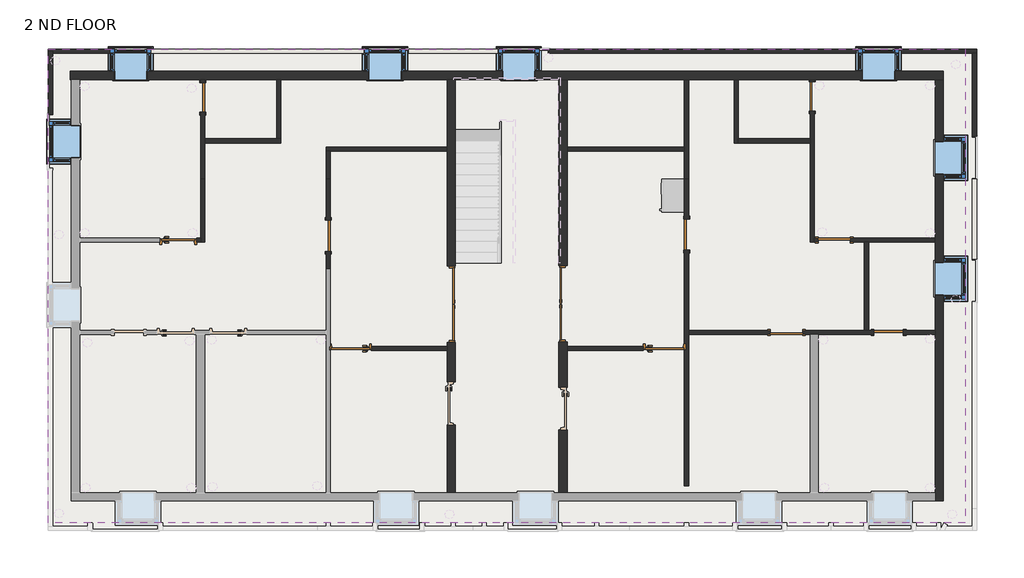
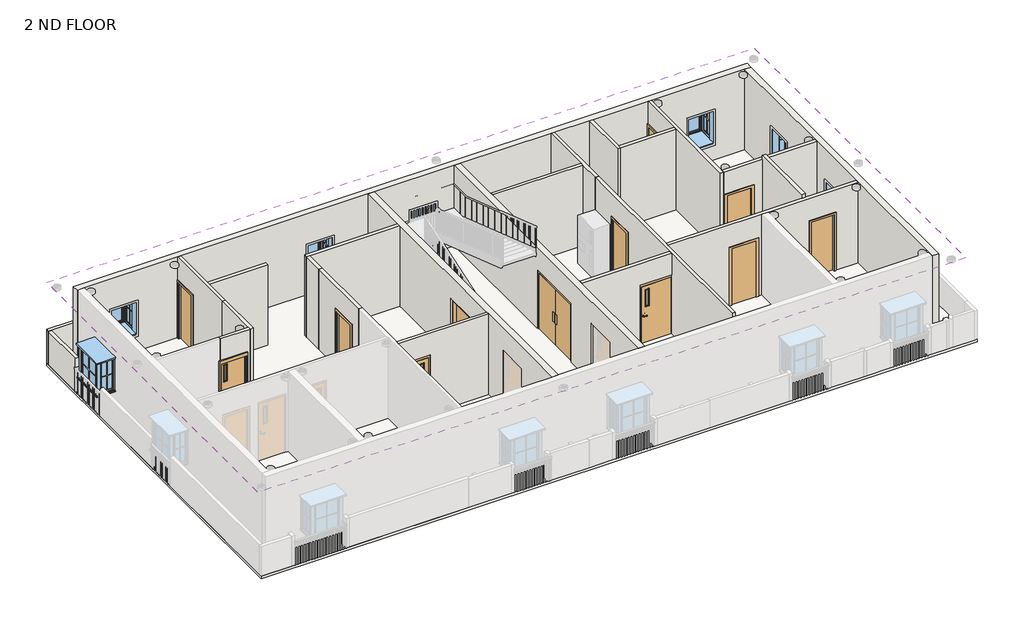
# One storey, part 2 of 7: 32 walls, 12 doors, 7 windows, 1 covering, 1 slab.
"""IFC4 building model written with IfcOpenShell, lengths in millimetres."""

from ifc_helpers import new_model, si_unit, frame, origin, place, context, project, spatial, polyline, outline, extrude, faceted_brep, transform, mapped, element, save
from components import door_2c854dd0, door_cf1f2706, door_4f5842df, door_passage_single_vision_lite_3_x7_440dd290, door_70e57c00, door_700d3439, door_8cb1b8a7, door_38851409, door_d141acb4, window_bay_casement_box_90_degree_angle_center_fixed_4_x3_2dea7aab

model = new_model("IFC4")

# Units and contexts
model_context = context("Model", 3, world=origin())
ifc_project = project(units=[si_unit("LENGTHUNIT", "METRE", prefix="MILLI")], contexts=[model_context])

# Site, building, storey
site = spatial("IfcSite", under=ifc_project)
building = spatial("IfcBuilding", under=site)
storey = spatial("IfcBuildingStorey", under=building, Name="2 ND FLOOR", Elevation=6400.8)

# Covering
placement = place(None, origin())
element("IfcCovering", 1, ObjectType="2' x 4' ACT System", at=placement, inside=storey, context=model_context, shape_type="SweptSolid", body=[
    extrude(outline(polyline([(12235.5012075, 8470.0067329), (12235.5012075, -4623.6932193), (-13088.8067989, -4623.6932193), (-13088.8067989, 8470.0067329), (12235.5012075, 8470.0067329)])), frame((0.0, 0.0, 9448.8), z_axis=(0.0, 0.0, 1.0), x_axis=(1.0, 0.0, 0.0)), (0.0, 0.0, 1.0), 57.15),
])

# Doors
door_shape = door_2c854dd0(model_context)
element("IfcDoor", 2, ObjectType="Door-Passage-Double-Flush-Dbl_Acting : 6'79\" X 84\"", at=placement, inside=storey, context=model_context, shape_type="MappedRepresentation", body=[
    mapped(door_shape, transform((-1969.4487998, 1424.4578621, 6400.8), x_axis=(0.0, -1.0, 0.0), y_axis=(1.0, 0.0, 0.0), z_axis=(0.0, 0.0, 1.0))),
])
element("IfcDoor", 3, ObjectType="Door-Passage-Double-Flush-Dbl_Acting : 6'79\" X 84\"", at=placement, inside=storey, context=model_context, shape_type="MappedRepresentation", body=[
    mapped(door_shape, transform((1128.8432011, 1434.2067807, 6400.8), x_axis=(0.0, 1.0, 0.0), y_axis=(-1.0, 0.0, 0.0), z_axis=(0.0, 0.0, 1.0))),
])
door_2_shape = door_cf1f2706(model_context)
element("IfcDoor", 4, ObjectType="Door-Passage-Single-Vision_Lite : 3'6\"X7' 2", at=placement, inside=storey, context=model_context, shape_type="MappedRepresentation", body=[
    mapped(door_2_shape, transform((-4750.7487995, 211.6078621, 6400.8), x_axis=(-1.0, 0.0, 0.0), y_axis=(0.0, -1.0, 0.0), z_axis=(0.0, 0.0, 1.0))),
])
door_3_shape = door_4f5842df(model_context)
element("IfcDoor", 5, ObjectType="Door-Passage-Single-Vision_Lite : 3'6\"X7' 2", at=placement, inside=storey, context=model_context, shape_type="MappedRepresentation", body=[
    mapped(door_3_shape, transform((3923.3512082, 211.6078621, 6400.8), x_axis=(1.0, 0.0, 0.0), y_axis=(0.0, 1.0, 0.0), z_axis=(0.0, 0.0, 1.0))),
])
door_passage_single_vision_lite_3_x7_shape = door_passage_single_vision_lite_3_x7_440dd290(model_context)
element("IfcDoor", 6, ObjectType="Door-Passage-Single-Vision_Lite : 3'X7'", at=placement, inside=storey, context=model_context, shape_type="MappedRepresentation", body=[
    mapped(door_passage_single_vision_lite_3_x7_shape, transform((-9501.8462614, 3186.8067332, 6400.8), x_axis=(1.0, 0.0, 0.0), y_axis=(0.0, 1.0, 0.0), z_axis=(0.0, 0.0, 1.0))),
])
door_4_shape = door_70e57c00(model_context)
element("IfcDoor", 7, ObjectType="Single-Flush : 2'10\" x 7'", at=placement, inside=storey, context=model_context, shape_type="MappedRepresentation", body=[
    mapped(door_4_shape, transform((-5360.3487995, 3313.8067802, 6400.8), x_axis=(0.0, -1.0, 0.0), y_axis=(1.0, 0.0, 0.0), z_axis=(0.0, 0.0, 1.0))),
])
door_5_shape = door_700d3439(model_context)
element("IfcDoor", 8, ObjectType="Single-Flush : 2'10\" x 7'", at=placement, inside=storey, context=model_context, shape_type="MappedRepresentation", body=[
    mapped(door_5_shape, transform((4532.9512082, 3351.906733, 6400.8), x_axis=(0.0, -1.0, 0.0), y_axis=(1.0, 0.0, 0.0), z_axis=(0.0, 0.0, 1.0))),
])
door_6_shape = door_8cb1b8a7(model_context)
element("IfcDoor", 9, ObjectType="Single-Flush : 2'11\"x 7'", at=placement, inside=storey, context=model_context, shape_type="MappedRepresentation", body=[
    mapped(door_6_shape, transform((8609.6512079, 3193.1567332, 6400.8), x_axis=(-1.0, 0.0, 0.0), y_axis=(0.0, -1.0, 0.0), z_axis=(0.0, 0.0, 1.0))),
])
element("IfcDoor", 10, ObjectType="Single-Flush : 2'11\"x 7'", at=placement, inside=storey, context=model_context, shape_type="MappedRepresentation", body=[
    mapped(door_6_shape, transform((7295.2012079, 640.4567334, 6400.8), x_axis=(1.0, 0.0, 0.0), y_axis=(0.0, 1.0, 0.0), z_axis=(0.0, 0.0, 1.0))),
])
door_7_shape = door_38851409(model_context)
element("IfcDoor", 11, ObjectType="Single-Flush : 2'8\"x 7'", at=placement, inside=storey, context=model_context, shape_type="MappedRepresentation", body=[
    mapped(door_7_shape, transform((-8827.4487992, 7136.5067329, 6400.8), x_axis=(0.0, 1.0, 0.0), y_axis=(-1.0, 0.0, 0.0), z_axis=(0.0, 0.0, 1.0))),
])
element("IfcDoor", 12, ObjectType="Single-Flush : 2'8\"x 7'", at=placement, inside=storey, context=model_context, shape_type="MappedRepresentation", body=[
    mapped(door_7_shape, transform((10111.5098918, 640.4567334, 6400.8), x_axis=(-1.0, 0.0, 0.0), y_axis=(0.0, -1.0, 0.0), z_axis=(0.0, 0.0, 1.0))),
])
door_8_shape = door_d141acb4(model_context)
element("IfcDoor", 13, ObjectType="Single-Flush : 2'8\"x 7'", at=placement, inside=storey, context=model_context, shape_type="MappedRepresentation", body=[
    mapped(door_8_shape, transform((8000.0512079, 7167.840939, 6400.8), x_axis=(0.0, 1.0, 0.0), y_axis=(-1.0, 0.0, 0.0), z_axis=(0.0, 0.0, 1.0))),
])

# Slab
element("IfcSlab", 14, ObjectType="LW Concrete on Metal Deck", at=placement, inside=storey, context=model_context, shape_type="SweptSolid", body=[
    extrude(outline(polyline([(12540.3012043, 8470.0067329), (12540.3012043, -4826.8932661), (-13088.8067989, -4826.8932661), (-13088.8067989, 8470.0067329), (12540.3012043, 8470.0067329)])), frame((0.0, 0.0, 6296.025), z_axis=(0.0, 0.0, 1.0), x_axis=(1.0, 0.0, 0.0)), (0.0, 0.0, 1.0), 104.775),
])

# Walls
element("IfcWall", 15, ObjectType="Generic - 4.5\"", at=placement, inside=storey, context=model_context, shape_type="Brep", body=[
    faceted_brep([(-8884.5987992, 4875.906733, 6400.8), (-8884.5987992, 3250.3067332, 6400.8), (-8884.5987992, 3136.0067332, 6400.8), (-8884.5987992, 3136.0067332, 9448.8), (-8884.5987992, 3250.3067332, 9448.8), (-8884.5987992, 4875.906733, 9448.8), (-8770.2987992, 4875.906733, 6400.8), (-8770.2987992, 4875.906733, 9448.8), (-8770.2987992, 3136.0067332, 9448.8), (-8770.2987992, 3136.0067332, 6400.8)], [[[0, 1, 2, 3, 4, 5]], [[6, 7, 8, 9]], [[2, 1, 0, 6, 9]], [[5, 4, 3, 8, 7]], [[0, 5, 7, 6]], [[3, 2, 9, 8]]]),
])
element("IfcWall", 16, ObjectType="Generic - 4.5\"", at=placement, inside=storey, context=model_context, shape_type="SweptSolid", body=[
    extrude(outline(polyline([(9448.8, -2077.3987998), (9448.8, -5303.1987995), (8636.0, -5303.1987995), (8636.0, -4166.5487995), (6400.8, -4166.5487995), (6400.8, -2077.3987998), (9448.8, -2077.3987998)])), frame((0.0, 148.1078621, 0.0), z_axis=(0.0, 1.0, 0.0), x_axis=(0.0, 0.0, 1.0)), (0.0, 0.0, 1.0), 114.3),
])
element("IfcWall", 17, ObjectType="Generic - 4.5\"", at=placement, inside=storey, context=model_context, shape_type="Brep", body=[
    faceted_brep([(-2077.3987998, 5764.9067329, 6400.8), (-5417.4987995, 5764.9067329, 6400.8), (-5417.4987995, 5764.9067329, 9448.8), (-2077.3987998, 5764.9067329, 9448.8), (-2077.3987998, 5650.6067329, 6400.8), (-2077.3987998, 5650.6067329, 9448.8), (-5303.1987995, 5650.6067329, 9448.8), (-5417.4987995, 5650.6067329, 9448.8), (-5417.4987995, 5650.6067329, 6400.8), (-5303.1987995, 5650.6067329, 6400.8)], [[[0, 1, 2, 3]], [[4, 5, 6, 7, 8, 9]], [[1, 0, 4, 9, 8]], [[3, 2, 7, 6, 5]], [[2, 1, 8, 7]], [[0, 3, 5, 4]]]),
])
element("IfcWall", 18, ObjectType="Generic - 4.5\"", at=placement, inside=storey, context=model_context, shape_type="SweptSolid", body=[
    extrude(outline(polyline([(-5417.4987995, 4875.90678), (-5417.4987995, 5650.6067329), (-5303.1987995, 5650.6067329), (-5303.1987995, 4875.90678), (-5417.4987995, 4875.90678)])), frame((0.0, 0.0, 6400.8), z_axis=(0.0, 0.0, 1.0), x_axis=(1.0, 0.0, 0.0)), (0.0, 0.0, 1.0), 3048.0),
])
element("IfcWall", 19, ObjectType="Generic - 4.5\"", at=placement, inside=storey, context=model_context, shape_type="SweptSolid", body=[
    extrude(outline(polyline([(4475.8012082, 5650.6067329), (1250.0012085, 5650.6067329), (1250.0012085, 5764.9067329), (4475.8012082, 5764.9067329), (4475.8012082, 5650.6067329)])), frame((0.0, 0.0, 6400.8), z_axis=(0.0, 0.0, 1.0), x_axis=(1.0, 0.0, 0.0)), (0.0, 0.0, 1.0), 3048.0),
])
element("IfcWall", 20, ObjectType="Generic - 4.5\"", at=placement, inside=storey, context=model_context, shape_type="Brep", body=[
    faceted_brep([(4475.8012082, 7631.8067329, 6400.8), (4475.8012082, 5764.9067329, 6400.8), (4475.8012082, 5650.6067329, 6400.8), (4475.8012082, 4875.906733, 6400.8), (4475.8012082, 4875.906733, 9448.8), (4475.8012082, 5650.6067329, 9448.8), (4475.8012082, 5764.9067329, 9448.8), (4475.8012082, 7631.8067329, 9448.8), (4590.1012082, 7631.8067329, 6400.8), (4590.1012082, 7631.8067329, 9448.8), (4590.1012082, 4875.906733, 9448.8), (4590.1012082, 4875.906733, 6400.8)], [[[0, 1, 2, 3, 4, 5, 6, 7]], [[8, 9, 10, 11]], [[3, 2, 1, 0, 8, 11]], [[4, 3, 11, 10]], [[7, 6, 5, 4, 10, 9]], [[0, 7, 9, 8]]]),
])
element("IfcWall", 21, ObjectType="Generic - 4.5\"", at=placement, inside=storey, context=model_context, shape_type="Brep", body=[
    faceted_brep([(4475.8012082, -3594.9932193, 6400.8), (4475.8012082, -3594.9932193, 9448.8), (4475.8012082, 148.1078621, 9448.8), (4475.8012082, 262.4078621, 9448.8), (4475.8012082, 4875.906733, 9448.8), (4475.8012082, 4875.906733, 6400.8), (4475.8012082, 3783.706733, 6400.8), (4475.8012082, 3783.706733, 8534.4), (4475.8012082, 2920.106733, 8534.4), (4475.8012082, 2920.106733, 6400.8), (4475.8012082, 262.4078621, 6400.8), (4475.8012082, 262.4078621, 8636.0), (4475.8012082, 148.1078621, 8636.0), (4475.8012082, 148.1078621, 6400.8), (4590.1012082, -3594.9932193, 9448.8), (4590.1012082, -3594.9932193, 6400.8), (4590.1012082, 583.3067334, 6400.8), (4590.1012082, 697.6067334, 6400.8), (4590.1012082, 2920.106733, 6400.8), (4590.1012082, 2920.106733, 8534.4), (4590.1012082, 3783.706733, 8534.4), (4590.1012082, 3783.706733, 6400.8), (4590.1012082, 4875.906733, 6400.8), (4590.1012082, 4875.906733, 9448.8), (4590.1012082, 697.6067334, 9448.8), (4590.1012082, 583.3067334, 9448.8), (4507.5512082, 148.1078621, 6400.8), (4507.5512082, 262.4078621, 6400.8), (4507.5512082, 148.1078621, 8636.0), (4507.5512082, 262.4078621, 8636.0)], [[[0, 1, 2, 3, 4, 5, 6, 7, 8, 9, 10, 11, 12, 13]], [[14, 15, 16, 17, 18, 19, 20, 21, 22, 23, 24, 25]], [[15, 0, 13, 26, 27, 10, 9, 18, 17, 16]], [[5, 22, 21, 6]], [[1, 0, 15, 14]], [[4, 3, 2, 1, 14, 25, 24, 23]], [[5, 4, 23, 22]], [[19, 18, 9, 8]], [[20, 19, 8, 7]], [[21, 20, 7, 6]], [[28, 26, 13, 12]], [[27, 29, 11, 10]], [[26, 28, 29, 27]], [[29, 28, 12, 11]]]),
])
element("IfcWall", 22, ObjectType="Generic - 4.5\"", at=placement, inside=storey, context=model_context, shape_type="Brep", body=[
    faceted_brep([(5847.401208, 7631.8067329, 6400.8), (5847.401208, 5879.2067329, 6400.8), (5847.401208, 5879.2067329, 9448.8), (5847.401208, 7631.8067329, 9448.8), (5961.701208, 7631.8067329, 6400.8), (5961.701208, 7631.8067329, 9448.8), (5961.701208, 5993.5067329, 9448.8), (5961.701208, 5879.2067329, 9448.8), (5961.701208, 5879.2067329, 6400.8), (5961.701208, 5993.5067329, 6400.8)], [[[0, 1, 2, 3]], [[4, 5, 6, 7, 8, 9]], [[1, 0, 4, 9, 8]], [[3, 2, 7, 6, 5]], [[0, 3, 5, 4]], [[2, 1, 8, 7]]]),
])
element("IfcWall", 23, ObjectType="Generic - 4.5\"", at=placement, inside=storey, context=model_context, shape_type="SweptSolid", body=[
    extrude(outline(polyline([(7942.9012079, 5879.2067329), (5961.701208, 5879.2067329), (5961.701208, 5993.5067329), (7942.9012079, 5993.5067329), (7942.9012079, 5879.2067329)])), frame((0.0, 0.0, 6400.8), z_axis=(0.0, 0.0, 1.0), x_axis=(1.0, 0.0, 0.0)), (0.0, 0.0, 1.0), 3048.0),
])
element("IfcWall", 24, ObjectType="Generic - 4.5\"", at=placement, inside=storey, context=model_context, shape_type="Brep", body=[
    faceted_brep([(7942.9012079, 7625.040939, 6400.8), (7942.9012079, 7574.240939, 6400.8), (7942.9012079, 7574.240939, 8534.4), (7942.9012079, 6761.440939, 8534.4), (7942.9012079, 6761.440939, 6400.8), (7942.9012079, 5993.5067329, 6400.8), (7942.9012079, 5879.2067329, 6400.8), (7942.9012079, 3136.0067332, 6400.8), (7942.9012079, 3136.0067332, 9448.8), (7942.9012079, 5879.2067329, 9448.8), (7942.9012079, 5993.5067329, 9448.8), (7942.9012079, 7625.040939, 9448.8), (8057.2012079, 7574.240939, 8534.4), (8057.2012079, 7574.240939, 6400.8), (8057.2012079, 7625.040939, 6400.8), (8057.2012079, 7625.040939, 9448.8), (8057.2012079, 3250.3067332, 9448.8), (8057.2012079, 3136.0067332, 9448.8), (8057.2012079, 3136.0067332, 6400.8), (8057.2012079, 3250.3067332, 6400.8), (8057.2012079, 6761.440939, 6400.8), (8057.2012079, 6761.440939, 8534.4)], [[[0, 1, 2, 3, 4, 5, 6, 7, 8, 9, 10, 11]], [[12, 13, 14, 15, 16, 17, 18, 19, 20, 21]], [[14, 13, 1, 0]], [[20, 19, 18, 7, 6, 5, 4]], [[11, 10, 9, 8, 17, 16, 15]], [[0, 11, 15, 14]], [[8, 7, 18, 17]], [[2, 1, 13, 12]], [[3, 2, 12, 21]], [[4, 3, 21, 20]]]),
])
element("IfcWall", 25, ObjectType="Generic - 4.5\"", at=placement, inside=storey, context=model_context, shape_type="Brep", body=[
    faceted_brep([(8165.1512079, 3250.3067332, 8534.4), (8165.1512079, 3250.3067332, 6400.8), (8057.2012079, 3250.3067332, 6400.8), (8057.2012079, 3250.3067332, 9448.8), (11397.3012075, 3250.3067332, 9448.8), (11397.3012075, 3250.3067332, 6400.8), (9054.1512079, 3250.3067332, 6400.8), (9054.1512079, 3250.3067332, 8534.4), (8057.2012079, 3136.0067332, 6400.8), (8165.1512079, 3136.0067332, 6400.8), (8165.1512079, 3136.0067332, 8534.4), (9054.1512079, 3136.0067332, 8534.4), (9054.1512079, 3136.0067332, 6400.8), (9438.4098918, 3136.0067332, 6400.8), (9565.4098918, 3136.0067332, 6400.8), (11397.3012075, 3136.0067332, 6400.8), (11397.3012075, 3136.0067332, 9448.8), (8057.2012079, 3136.0067332, 9448.8)], [[[0, 1, 2, 3, 4, 5, 6, 7]], [[8, 9, 10, 11, 12, 13, 14, 15, 16, 17]], [[6, 5, 15, 14, 13, 12]], [[2, 1, 9, 8]], [[4, 3, 17, 16]], [[3, 2, 8, 17]], [[5, 4, 16, 15]], [[10, 9, 1, 0]], [[11, 10, 0, 7]], [[12, 11, 7, 6]]]),
])
element("IfcWall", 26, ObjectType="Generic - 4.5\"", at=placement, inside=storey, context=model_context, shape_type="Brep", body=[
    faceted_brep([(7739.7012079, 583.3067334, 8534.4), (7739.7012079, 583.3067334, 6400.8), (7942.9012079, 583.3067334, 6400.8), (8171.5012079, 583.3067334, 6400.8), (9705.1098918, 583.3067334, 6400.8), (9705.1098918, 583.3067334, 8534.4), (10517.9098918, 583.3067334, 8534.4), (10517.9098918, 583.3067334, 6400.8), (11397.3012075, 583.3067334, 6400.8), (11397.3012075, 583.3067334, 9448.8), (8171.5012079, 583.3067334, 9448.8), (7942.9012079, 583.3067334, 9448.8), (4590.1012082, 583.3067334, 9448.8), (4590.1012082, 583.3067334, 6400.8), (6850.7012079, 583.3067334, 6400.8), (6850.7012079, 583.3067334, 8534.4), (9705.1098918, 697.6067334, 6400.8), (9565.4098918, 697.6067334, 6400.8), (9438.4098918, 697.6067334, 6400.8), (7739.7012079, 697.6067334, 6400.8), (7739.7012079, 697.6067334, 8534.4), (6850.7012079, 697.6067334, 8534.4), (6850.7012079, 697.6067334, 6400.8), (4590.1012082, 697.6067334, 6400.8), (4590.1012082, 697.6067334, 9448.8), (11397.3012075, 697.6067334, 9448.8), (11397.3012075, 697.6067334, 6400.8), (10517.9098918, 697.6067334, 6400.8), (10517.9098918, 697.6067334, 8534.4), (9705.1098918, 697.6067334, 8534.4)], [[[0, 1, 2, 3, 4, 5, 6, 7, 8, 9, 10, 11, 12, 13, 14, 15]], [[16, 17, 18, 19, 20, 21, 22, 23, 24, 25, 26, 27, 28, 29]], [[27, 26, 8, 7]], [[14, 13, 23, 22]], [[4, 3, 2, 1, 19, 18, 17, 16]], [[12, 11, 10, 9, 25, 24]], [[9, 8, 26, 25]], [[13, 12, 24, 23]], [[5, 4, 16, 29]], [[6, 5, 29, 28]], [[7, 6, 28, 27]], [[20, 19, 1, 0]], [[21, 20, 0, 15]], [[22, 21, 15, 14]]]),
])
element("IfcWall", 27, ObjectType="Generic - 4.5\"", at=placement, inside=storey, context=model_context, shape_type="Brep", body=[
    faceted_brep([(-8770.2987992, 7542.9067329, 8534.4), (-8770.2987992, 7542.9067329, 6400.8), (-8770.2987992, 7631.8067329, 6400.8), (-8770.2987992, 7631.8067329, 9448.8), (-8770.2987992, 5993.5067329, 9448.8), (-8770.2987992, 5879.2067329, 9448.8), (-8770.2987992, 4875.906733, 9448.8), (-8770.2987992, 4875.906733, 6400.8), (-8770.2987992, 5879.2067329, 6400.8), (-8770.2987992, 5993.5067329, 6400.8), (-8770.2987992, 6730.1067329, 6400.8), (-8770.2987992, 6730.1067329, 8534.4), (-8884.5987992, 7631.8067329, 6400.8), (-8884.5987992, 7542.9067329, 6400.8), (-8884.5987992, 7542.9067329, 8534.4), (-8884.5987992, 6730.1067329, 8534.4), (-8884.5987992, 6730.1067329, 6400.8), (-8884.5987992, 4875.906733, 6400.8), (-8884.5987992, 4875.906733, 9448.8), (-8884.5987992, 7631.8067329, 9448.8)], [[[0, 1, 2, 3, 4, 5, 6, 7, 8, 9, 10, 11]], [[12, 13, 14, 15, 16, 17, 18, 19]], [[2, 1, 13, 12]], [[10, 9, 8, 7, 17, 16]], [[6, 5, 4, 3, 19, 18]], [[7, 6, 18, 17]], [[3, 2, 12, 19]], [[14, 13, 1, 0]], [[15, 14, 0, 11]], [[16, 15, 11, 10]]]),
])
element("IfcWall", 28, ObjectType="Generic - 4.5\"", at=placement, inside=storey, context=model_context, shape_type="Brep", body=[
    faceted_brep([(-8770.2987992, 5879.2067329, 6400.8), (-6674.7987994, 5879.2067329, 6400.8), (-6674.7987994, 5879.2067329, 9448.8), (-8770.2987992, 5879.2067329, 9448.8), (-8770.2987992, 5993.5067329, 6400.8), (-8770.2987992, 5993.5067329, 9448.8), (-6674.7987994, 5993.5067329, 9448.8), (-6674.7987994, 5993.5067329, 7772.4), (-6674.7987994, 5993.5067329, 6400.8), (-6789.0987994, 5993.5067329, 6400.8)], [[[0, 1, 2, 3]], [[4, 5, 6, 7, 8, 9]], [[1, 0, 4, 9, 8]], [[3, 2, 6, 5]], [[0, 3, 5, 4]], [[2, 1, 8, 7, 6]]]),
])
element("IfcWall", 29, ObjectType="Generic - 4.5\"", at=placement, inside=storey, context=model_context, shape_type="SweptSolid", body=[
    extrude(outline(polyline([(-6674.7987994, 7631.8067329), (-6674.7987994, 5993.5067329), (-6789.0987994, 5993.5067329), (-6789.0987994, 7631.8067329), (-6674.7987994, 7631.8067329)])), frame((0.0, 0.0, 6400.8), z_axis=(0.0, 0.0, 1.0), x_axis=(1.0, 0.0, 0.0)), (0.0, 0.0, 1.0), 1371.6),
])
element("IfcWall", 30, ObjectType="Generic - 4.5\"", at=placement, inside=storey, context=model_context, shape_type="SweptSolid", body=[
    extrude(outline(polyline([(9448.8, -8884.5987992), (9448.8, -9959.0462614), (8636.0, -9959.0462614), (8636.0, -8993.8462614), (6400.8, -8993.8462614), (6400.8, -8884.5987992), (9448.8, -8884.5987992)])), frame((0.0, 3136.0067332, 0.0), z_axis=(0.0, 1.0, 0.0), x_axis=(0.0, 0.0, 1.0)), (0.0, 0.0, 1.0), 114.3),
])
element("IfcWall", 31, ObjectType="Generic - 4.5\"", at=placement, inside=storey, context=model_context, shape_type="SweptSolid", body=[
    extrude(outline(polyline([(2882.0067802, 8534.4), (2882.0067802, 6400.8), (2399.4067802, 6400.8), (2399.4067802, 9448.8), (4875.90678, 9448.8), (4875.90678, 6400.8), (3745.6067802, 6400.8), (3745.6067802, 8534.4), (2882.0067802, 8534.4)])), frame((-5417.4987995, 0.0, 0.0), z_axis=(1.0, 0.0, 0.0), x_axis=(0.0, 1.0, 0.0)), (0.0, 0.0, 1.0), 114.3),
])
element("IfcWall", 32, ObjectType="Generic - 4.5\"", at=placement, inside=storey, context=model_context, shape_type="SweptSolid", body=[
    extrude(outline(polyline([(9448.8, 4475.8012082), (9448.8, 1250.0012085), (6400.8, 1250.0012085), (6400.8, 3339.1512082), (8636.0, 3339.1512082), (8636.0, 4475.8012082), (9448.8, 4475.8012082)])), frame((0.0, 148.1078621, 0.0), z_axis=(0.0, 1.0, 0.0), x_axis=(0.0, 0.0, 1.0)), (0.0, 0.0, 1.0), 114.3),
])
element("IfcWall", 33, ObjectType="Generic - 4.5\"", at=placement, inside=storey, context=model_context, shape_type="SweptSolid", body=[
    extrude(outline(polyline([(-12973.9987925, 8412.8567329), (-12973.9987925, 6682.2711337), (-13088.2987925, 6682.2711337), (-13088.2987925, 8412.8567329), (-12973.9987925, 8412.8567329)])), frame((0.0, 0.0, 6400.8), z_axis=(0.0, 0.0, 1.0), x_axis=(1.0, 0.0, 0.0)), (0.0, 0.0, 1.0), 1259.0059812),
])
element("IfcWall", 34, ObjectType="Generic - 4.5\"", at=placement, inside=storey, context=model_context, shape_type="SweptSolid", body=[
    extrude(outline(polyline([(-11387.0067989, 8355.7067329), (-13088.8067989, 8355.7067329), (-13088.8067989, 8470.0067329), (-11387.0067989, 8470.0067329), (-11387.0067989, 8355.7067329)])), frame((0.0, 0.0, 6400.8), z_axis=(0.0, 0.0, 1.0), x_axis=(1.0, 0.0, 0.0)), (0.0, 0.0, 1.0), 1273.4134002),
])
element("IfcWall", 35, ObjectType="Generic - 4.5\"", at=placement, inside=storey, context=model_context, shape_type="SweptSolid", body=[
    extrude(outline(polyline([(-4382.4487992, 8355.7067329), (-10247.1817989, 8355.7067329), (-10247.1817989, 8470.0067329), (-4382.4487992, 8470.0067329), (-4382.4487992, 8355.7067329)])), frame((0.0, 0.0, 6400.8), z_axis=(0.0, 0.0, 1.0), x_axis=(1.0, 0.0, 0.0)), (0.0, 0.0, 1.0), 1083.89837),
])
element("IfcWall", 36, ObjectType="Generic - 4.5\"", at=placement, inside=storey, context=model_context, shape_type="SweptSolid", body=[
    extrude(outline(polyline([(-682.0490672, 8355.7067329), (-3139.4990672, 8355.7067329), (-3139.4990672, 8470.0067329), (-682.0490672, 8470.0067329), (-682.0490672, 8355.7067329)])), frame((0.0, 0.0, 6400.8), z_axis=(0.0, 0.0, 1.0), x_axis=(1.0, 0.0, 0.0)), (0.0, 0.0, 1.0), 1195.9732529),
])
element("IfcWall", 37, ObjectType="Generic - 4.5\"", at=placement, inside=storey, context=model_context, shape_type="SweptSolid", body=[
    extrude(outline(polyline([(9199.6932011, 8355.7067329), (741.4932011, 8355.7067329), (741.4932011, 8470.0067329), (9199.6932011, 8470.0067329), (9199.6932011, 8355.7067329)])), frame((0.0, 0.0, 6400.8), z_axis=(0.0, 0.0, 1.0), x_axis=(1.0, 0.0, 0.0)), (0.0, 0.0, 1.0), 1274.1868366),
])
element("IfcWall", 38, ObjectType="Generic - 4.5\"", at=placement, inside=storey, context=model_context, shape_type="Brep", body=[
    faceted_brep([(10462.2009401, 8355.7067329, 6400.8), (12426.0012043, 8355.7067329, 6400.8), (12540.3012043, 8355.7067329, 6400.8), (12540.3012043, 8355.7067329, 7766.5502881), (10462.2009401, 8355.7067329, 7766.5502881), (10462.2009401, 8470.0067329, 6400.8), (10462.2009401, 8470.0067329, 7766.5502881), (12540.3012043, 8470.0067329, 7766.5502881), (12540.3012043, 8470.0067329, 6400.8)], [[[0, 1, 2, 3, 4]], [[5, 6, 7, 8]], [[2, 1, 0, 5, 8]], [[4, 3, 7, 6]], [[0, 4, 6, 5]], [[3, 2, 8, 7]]]),
])
element("IfcWall", 39, ObjectType="Generic - 4.5\"", at=placement, inside=storey, context=model_context, shape_type="Brep", body=[
    faceted_brep([(12426.0012043, 8355.7067329, 6400.8), (12426.0012043, 6069.7067329, 6400.8), (12426.0012043, 6069.7067329, 7772.4), (12426.0012043, 8355.7067329, 7772.4), (12540.3012043, 8355.7067329, 6400.8), (12540.3012043, 8355.7067329, 7766.5502881), (12540.3012043, 8355.7067329, 7772.4), (12540.3012043, 6069.7067329, 7772.4), (12540.3012043, 6069.7067329, 6400.8)], [[[0, 1, 2, 3]], [[4, 5, 6, 7, 8]], [[1, 0, 4, 8]], [[2, 1, 8, 7]], [[3, 2, 7, 6]], [[0, 3, 6, 5, 4]]]),
])
element("IfcWall", 40, ObjectType="Generic - 4.5\"", at=placement, inside=storey, context=model_context, shape_type="SweptSolid", body=[
    extrude(outline(polyline([(12426.0012043, 2666.1067329), (12426.0012043, 4875.9067329), (12540.3012043, 4875.9067329), (12540.3012043, 2666.1067329), (12426.0012043, 2666.1067329)])), frame((0.0, 0.0, 6400.8), z_axis=(0.0, 0.0, 1.0), x_axis=(1.0, 0.0, 0.0)), (0.0, 0.0, 1.0), 1193.0409005),
])
element("IfcWall", 41, ObjectType="Generic - 9\"", at=placement, inside=storey, context=model_context, shape_type="Brep", body=[
    faceted_brep([(-12479.2067989, 7631.8067329, 6400.8), (-12453.2987925, 7631.8067329, 6400.8), (-12224.6987925, 7631.8067329, 6400.8), (-8884.5987992, 7631.8067329, 6400.8), (-8770.2987992, 7631.8067329, 6400.8), (-6789.0987994, 7631.8067329, 6400.8), (-6674.7987994, 7631.8067329, 6400.8), (-2077.3987998, 7631.8067329, 6400.8), (-1848.7987998, 7631.8067329, 6400.8), (1008.1932011, 7631.8067329, 6400.8), (1236.7932011, 7631.8067329, 6400.8), (4475.8012082, 7631.8067329, 6400.8), (4590.1012082, 7631.8067329, 6400.8), (5847.401208, 7631.8067329, 6400.8), (5961.701208, 7631.8067329, 6400.8), (11397.3012075, 7631.8067329, 6400.8), (11625.9012075, 7631.8067329, 6400.8), (11625.9012075, 7631.8067329, 9448.8), (11397.3012075, 7631.8067329, 9448.8), (5961.701208, 7631.8067329, 9448.8), (5847.401208, 7631.8067329, 9448.8), (4590.1012082, 7631.8067329, 9448.8), (4475.8012082, 7631.8067329, 9448.8), (1236.7932011, 7631.8067329, 9448.8), (1008.1932011, 7631.8067329, 9448.8), (-1848.7987998, 7631.8067329, 9448.8), (-2077.3987998, 7631.8067329, 9448.8), (-8770.2987992, 7631.8067329, 9448.8), (-8884.5987992, 7631.8067329, 9448.8), (-12224.6987925, 7631.8067329, 9448.8), (-12453.2987925, 7631.8067329, 9448.8), (-12479.2067989, 7631.8067329, 9448.8), (-10357.7987925, 7631.8067329, 8280.4), (-10357.7987925, 7631.8067329, 7010.4), (-11272.1987925, 7631.8067329, 7010.4), (-11272.1987925, 7631.8067329, 8280.4), (-3334.6987998, 7631.8067329, 8280.4), (-3334.6987998, 7631.8067329, 7010.4), (-4249.0987998, 7631.8067329, 7010.4), (-4249.0987998, 7631.8067329, 8280.4), (360.4932011, 7631.8067329, 8280.4), (360.4932011, 7631.8067329, 7010.4), (-553.9067989, 7631.8067329, 7010.4), (-553.9067989, 7631.8067329, 8280.4), (10292.4012075, 7631.8067329, 8280.4), (10292.4012075, 7631.8067329, 7010.4), (9378.0012075, 7631.8067329, 7010.4), (9378.0012075, 7631.8067329, 8280.4), (-12479.2067989, 7860.4067329, 6400.8), (-12479.2067989, 7860.4067329, 9448.8), (11625.9012075, 7860.4067329, 9448.8), (11625.9012075, 7860.4067329, 6400.8), (-10357.7987925, 7860.4067329, 8280.4), (-11272.1987925, 7860.4067329, 8280.4), (-11272.1987925, 7860.4067329, 7010.4), (-10357.7987925, 7860.4067329, 7010.4), (-3334.6987998, 7860.4067329, 8280.4), (-4249.0987998, 7860.4067329, 8280.4), (-4249.0987998, 7860.4067329, 7010.4), (-3334.6987998, 7860.4067329, 7010.4), (360.4932011, 7860.4067329, 8280.4), (-553.9067989, 7860.4067329, 8280.4), (-553.9067989, 7860.4067329, 7010.4), (360.4932011, 7860.4067329, 7010.4), (10292.4012075, 7860.4067329, 8280.4), (9378.0012075, 7860.4067329, 8280.4), (9378.0012075, 7860.4067329, 7010.4), (10292.4012075, 7860.4067329, 7010.4)], [[[0, 1, 2, 3, 4, 5, 6, 7, 8, 9, 10, 11, 12, 13, 14, 15, 16, 17, 18, 19, 20, 21, 22, 23, 24, 25, 26, 27, 28, 29, 30, 31], [32, 33, 34, 35], [36, 37, 38, 39], [40, 41, 42, 43], [44, 45, 46, 47]], [[48, 49, 50, 51], [52, 53, 54, 55], [56, 57, 58, 59], [60, 61, 62, 63], [64, 65, 66, 67]], [[16, 15, 14, 13, 12, 11, 10, 9, 8, 7, 6, 5, 4, 3, 2, 1, 0, 48, 51]], [[31, 30, 29, 28, 27, 26, 25, 24, 23, 22, 21, 20, 19, 18, 17, 50, 49]], [[0, 31, 49, 48]], [[17, 16, 51, 50]], [[33, 32, 52, 55]], [[34, 33, 55, 54]], [[35, 34, 54, 53]], [[32, 35, 53, 52]], [[37, 36, 56, 59]], [[38, 37, 59, 58]], [[39, 38, 58, 57]], [[36, 39, 57, 56]], [[41, 40, 60, 63]], [[42, 41, 63, 62]], [[43, 42, 62, 61]], [[40, 43, 61, 60]], [[45, 44, 64, 67]], [[46, 45, 67, 66]], [[47, 46, 66, 65]], [[44, 47, 65, 64]]]),
])
element("IfcWall", 42, ObjectType="Generic - 9\"", at=placement, inside=storey, context=model_context, shape_type="Brep", body=[
    faceted_brep([(11397.3012075, 7631.8067329, 6400.8), (11397.3012075, 3250.3067332, 6400.8), (11397.3012075, 3136.0067332, 6400.8), (11397.3012075, 697.6067334, 6400.8), (11397.3012075, 583.3067334, 6400.8), (11397.3012075, -3785.4932193, 6400.8), (11397.3012075, -4014.0932193, 6400.8), (11397.3012075, -4014.0932193, 9448.8), (11397.3012075, -3785.4932193, 9448.8), (11397.3012075, 583.3067334, 9448.8), (11397.3012075, 697.6067334, 9448.8), (11397.3012075, 3136.0067332, 9448.8), (11397.3012075, 3250.3067332, 9448.8), (11397.3012075, 7631.8067329, 9448.8), (11397.3012075, 1669.1567332, 8280.4), (11397.3012075, 1669.1567332, 7010.4), (11397.3012075, 2583.5567332, 7010.4), (11397.3012075, 2583.5567332, 8280.4), (11397.3012075, 5012.431733, 8280.4), (11397.3012075, 5012.431733, 7010.4), (11397.3012075, 5926.831733, 7010.4), (11397.3012075, 5926.831733, 8280.4), (11625.9012075, 7631.8067329, 6400.8), (11625.9012075, 7631.8067329, 9448.8), (11625.9012075, -4014.0932193, 9448.8), (11625.9012075, -4014.0932193, 6400.8), (11625.9012075, 1669.1567332, 8280.4), (11625.9012075, 2583.5567332, 8280.4), (11625.9012075, 2583.5567332, 7010.4), (11625.9012075, 1669.1567332, 7010.4), (11625.9012075, 5012.431733, 8280.4), (11625.9012075, 5926.831733, 8280.4), (11625.9012075, 5926.831733, 7010.4), (11625.9012075, 5012.431733, 7010.4)], [[[0, 1, 2, 3, 4, 5, 6, 7, 8, 9, 10, 11, 12, 13], [14, 15, 16, 17], [18, 19, 20, 21]], [[22, 23, 24, 25], [26, 27, 28, 29], [30, 31, 32, 33]], [[6, 5, 4, 3, 2, 1, 0, 22, 25]], [[13, 12, 11, 10, 9, 8, 7, 24, 23]], [[0, 13, 23, 22]], [[7, 6, 25, 24]], [[15, 14, 26, 29]], [[16, 15, 29, 28]], [[17, 16, 28, 27]], [[14, 17, 27, 26]], [[19, 18, 30, 33]], [[20, 19, 33, 32]], [[21, 20, 32, 31]], [[18, 21, 31, 30]]]),
])
element("IfcWall", 43, ObjectType="Generic - 9\"", at=placement, inside=storey, context=model_context, shape_type="Brep", body=[
    faceted_brep([(-2077.3987998, -3785.4932193, 9448.8), (-2077.3987998, 148.1078621, 9448.8), (-2077.3987998, 262.4078621, 9448.8), (-2077.3987998, 5650.6067329, 9448.8), (-2077.3987998, 5764.9067329, 9448.8), (-2077.3987998, 7631.8067329, 9448.8), (-2077.3987998, 7631.8067329, 6400.8), (-2077.3987998, 5764.9067329, 6400.8), (-2077.3987998, 5650.6067329, 6400.8), (-2077.3987998, 2478.5578621, 6400.8), (-2077.3987998, 2478.5578621, 8636.0), (-2077.3987998, 370.3578621, 8636.0), (-2077.3987998, 370.3578621, 6400.8), (-2077.3987998, 262.4078621, 6400.8), (-2077.3987998, 148.1078621, 6400.8), (-2077.3987998, -721.8421379, 6400.8), (-2077.3987998, -721.8421379, 8636.0), (-2077.3987998, -1915.6421379, 8636.0), (-2077.3987998, -1915.6421379, 6400.8), (-2077.3987998, -3785.4932193, 6400.8), (-1848.7987998, 7631.8067329, 9448.8), (-1848.7987998, -3785.4932193, 9448.8), (-1848.7987998, -3785.4932193, 6400.8), (-1848.7987998, -1915.6421379, 6400.8), (-1848.7987998, -1915.6421379, 8636.0), (-1848.7987998, -721.8421379, 8636.0), (-1848.7987998, -721.8421379, 6400.8), (-1848.7987998, 370.3578621, 6400.8), (-1848.7987998, 370.3578621, 8636.0), (-1848.7987998, 2478.5578621, 8636.0), (-1848.7987998, 2478.5578621, 6400.8), (-1848.7987998, 7631.8067329, 6400.8)], [[[0, 1, 2, 3, 4, 5, 6, 7, 8, 9, 10, 11, 12, 13, 14, 15, 16, 17, 18, 19]], [[20, 21, 22, 23, 24, 25, 26, 27, 28, 29, 30, 31]], [[22, 19, 18, 23]], [[6, 31, 30, 9, 8, 7]], [[26, 15, 14, 13, 12, 27]], [[5, 4, 3, 2, 1, 0, 21, 20]], [[0, 19, 22, 21]], [[6, 5, 20, 31]], [[17, 24, 23, 18]], [[24, 17, 16, 25]], [[25, 16, 15, 26]], [[11, 28, 27, 12]], [[28, 11, 10, 29]], [[29, 10, 9, 30]]]),
])
element("IfcWall", 44, ObjectType="Generic - 9\"", at=placement, inside=storey, context=model_context, shape_type="SweptSolid", body=[
    extrude(outline(polyline([(-3785.4932193, 9448.8), (7631.8067329, 9448.8), (7631.8067329, 6400.8), (2488.3067807, 6400.8), (2488.3067807, 8636.0), (380.1067807, 8636.0), (380.1067807, 6400.8), (-877.1932193, 6400.8), (-877.1932193, 8636.0), (-2045.5932193, 8636.0), (-2045.5932193, 6400.8), (-3785.4932193, 6400.8), (-3785.4932193, 9448.8)])), frame((1008.1932011, 0.0, 0.0), z_axis=(1.0, 0.0, 0.0), x_axis=(0.0, 1.0, 0.0)), (0.0, 0.0, 1.0), 228.6),
])
element("IfcWall", 45, ObjectType="Interior - 5\" Partition (2-hr)", at=placement, inside=storey, context=model_context, shape_type="SweptSolid", body=[
    extrude(outline(polyline([(9438.4098918, 697.6067334), (9438.4098918, 3136.0067332), (9565.4098918, 3136.0067332), (9565.4098918, 697.6067334), (9438.4098918, 697.6067334)])), frame((0.0, 0.0, 6400.8), z_axis=(0.0, 0.0, 1.0), x_axis=(1.0, 0.0, 0.0)), (0.0, 0.0, 1.0), 3200.4),
])
element("IfcWall", 46, ObjectType="Interior - 5\" Partition (2-hr)", at=placement, inside=storey, context=model_context, shape_type="SweptSolid", body=[
    extrude(outline(polyline([(9438.4098918, 697.6067334), (9438.4098918, 3136.0067332), (9565.4098918, 3136.0067332), (9565.4098918, 697.6067334), (9438.4098918, 697.6067334)])), frame((0.0, 0.0, 6400.8), z_axis=(0.0, 0.0, 1.0), x_axis=(1.0, 0.0, 0.0)), (0.0, 0.0, 1.0), 3200.4),
])

# Windows
window_bay_casement_box_90_degree_angle_center_fixed_4_x3_shape = window_bay_casement_box_90_degree_angle_center_fixed_4_x3_2dea7aab(model_context)
element("IfcWindow", 47, ObjectType="Window-Bay-Casement-Box-90_Degree_Angle-Center_Fixed : 4'X3'", at=placement, inside=storey, context=model_context, shape_type="MappedRepresentation", body=[
    mapped(window_bay_casement_box_90_degree_angle_center_fixed_4_x3_shape, transform((-10814.9987925, 7746.1067329, 6400.8), x_axis=(1.0, 0.0, 0.0), y_axis=(0.0, 1.0, 0.0), z_axis=(0.0, 0.0, 1.0))),
])
element("IfcWindow", 48, ObjectType="Window-Bay-Casement-Box-90_Degree_Angle-Center_Fixed : 4'X3'", at=placement, inside=storey, context=model_context, shape_type="MappedRepresentation", body=[
    mapped(window_bay_casement_box_90_degree_angle_center_fixed_4_x3_shape, transform((-3791.8987998, 7746.1067329, 6400.8), x_axis=(1.0, 0.0, 0.0), y_axis=(0.0, 1.0, 0.0), z_axis=(0.0, 0.0, 1.0))),
])
element("IfcWindow", 49, ObjectType="Window-Bay-Casement-Box-90_Degree_Angle-Center_Fixed : 4'X3'", at=placement, inside=storey, context=model_context, shape_type="MappedRepresentation", body=[
    mapped(window_bay_casement_box_90_degree_angle_center_fixed_4_x3_shape, transform((-96.7067989, 7746.1067329, 6400.8), x_axis=(1.0, 0.0, 0.0), y_axis=(0.0, 1.0, 0.0), z_axis=(0.0, 0.0, 1.0))),
])
element("IfcWindow", 50, ObjectType="Window-Bay-Casement-Box-90_Degree_Angle-Center_Fixed : 4'X3'", at=placement, inside=storey, context=model_context, shape_type="MappedRepresentation", body=[
    mapped(window_bay_casement_box_90_degree_angle_center_fixed_4_x3_shape, transform((9835.2012075, 7746.1067329, 6400.8), x_axis=(1.0, 0.0, 0.0), y_axis=(0.0, 1.0, 0.0), z_axis=(0.0, 0.0, 1.0))),
])
element("IfcWindow", 51, ObjectType="Window-Bay-Casement-Box-90_Degree_Angle-Center_Fixed : 4'X3'", at=placement, inside=storey, context=model_context, shape_type="MappedRepresentation", body=[
    mapped(window_bay_casement_box_90_degree_angle_center_fixed_4_x3_shape, transform((11511.6012075, 2126.3567332, 6400.8), x_axis=(0.0, -1.0, 0.0), y_axis=(1.0, 0.0, 0.0), z_axis=(0.0, 0.0, 1.0))),
])
element("IfcWindow", 52, ObjectType="Window-Bay-Casement-Box-90_Degree_Angle-Center_Fixed : 4'X3'", at=placement, inside=storey, context=model_context, shape_type="MappedRepresentation", body=[
    mapped(window_bay_casement_box_90_degree_angle_center_fixed_4_x3_shape, transform((11511.6012075, 5469.631733, 6400.8), x_axis=(0.0, -1.0, 0.0), y_axis=(1.0, 0.0, 0.0), z_axis=(0.0, 0.0, 1.0))),
])
element("IfcWindow", 53, ObjectType="Window-Bay-Casement-Box-90_Degree_Angle-Center_Fixed : 4'X3'", at=placement, inside=storey, context=model_context, shape_type="MappedRepresentation", body=[
    mapped(window_bay_casement_box_90_degree_angle_center_fixed_4_x3_shape, transform((-12338.9987925, 5917.3067329, 6400.8), x_axis=(0.0, 1.0, 0.0), y_axis=(-1.0, 0.0, 0.0), z_axis=(0.0, 0.0, 1.0))),
])

save(model, "model.ifc")

# Revit data of these elements
# Type "2' x 4' ACT System"
#   Assembly Code = "C3030210"
#   built-in parameter 1002203 = 1 (stored number, unit not read)
#   built-in parameter 1002202 = 1 (stored number, unit not read)
#   Layers, outside or top first: 0' - 1 5/8" "Default" (function 1); 0' - 0 5/8" "Acoustic Ceiling Tile 24 x 48" (function 5)
# Type "Door-Passage-Double-Flush-Dbl_Acting : 6'79\" X 84\""
#   Type Mark = "17"
#   Assembly Code = "B2030200"
#   Analytic Construction = "Metal"
#   W = 3' - 3 1/2"
#   Thickness = 0' - 1 3/4"
#   Thermal Resistance (R) = 1.5338 (h·ft²·°F)/BTU
#   Swing Angle [instance default] = 90.00°
#   Strike Height = 3' - 4"
#   Single Panel Width = 3' - 3 1/2"
#   Rough Width [instance default] = 6' - 11"
#   Rough Height [instance default] = 7' - 4"
#   MF Opening Height [instance default] = 0' - 4"
#   MF Opening Width [instance default] = 0' - 4"
#   Inset Calculate [instance default] = 0' - 4"
#   Masonry Inset [instance default] = 0' - 1"
#   Height = 7' - 0"
#   Width = 6' - 7"
#   Heat Transfer Coefficient (U) = 0.6520 BTU/(h·ft²·°F)
#   Masonry Frame Depth = 0' - 5 3/4"
#   Masonry Frame [instance default] = yes
#   Function = 1
#   Dry Wall Frame [instance default] = no
#   Panel Material = Metal - Paint Finish - Brindle
#   Frame Material = Metal - Paint Finish - Grey
#   Door Handle Material = Aluminium
#   Visual Light Transmittance = 0
#   Solar Heat Gain Coefficient = 0
#   Wall Closure = (empty or 0)
# Type "Door-Passage-Single-Vision_Lite : 3'6\"X7' 2"
#   Type Mark = "14"
#   Assembly Code = "B2030100"
#   Analytic Construction = "Wooden"
#   Thickness = 0' - 1 3/4"
#   Thermal Resistance (R) = 2.5876 (h·ft²·°F)/BTU
#   Swing Angle [instance default] = 90.00°
#   Strike Height = 3' - 4"
#   Rough Width [instance default] = 3' - 10"
#   Rough Height [instance default] = 7' - 4"
#   MFOpeningHeight [instance default] = 0' - 4"
#   MFOpeningWidth [instance default] = 0' - 4"
#   Inset Calculate [instance default] = 0' - 4"
#   Masonry Inset [instance default] = 0' - 1"
#   Height = 7' - 0"
#   Width = 3' - 6"
#   Heat Transfer Coefficient (U) = 0.3865 BTU/(h·ft²·°F)
#   Masonry Frame Depth = 0' - 5 3/4"
#   Masonry Frame [instance default] = yes
#   Function = 1
#   Dry Wall Frame [instance default] = no
#   Panel Material = Wood - Birch
#   Glazing = Glass
#   Glass Stop Material = Metal - Paint Finish - Grey
#   Frame Material = Metal - Paint Finish - Grey
#   Door Handle Material = Aluminum
#   Visual Light Transmittance = 0
#   Solar Heat Gain Coefficient = 0
#   Wall Closure = (empty or 0)
# Type "Door-Passage-Single-Vision_Lite : 3'X7'"
#   Type Mark = "9"
#   Assembly Code = "B2030100"
#   Analytic Construction = "Wooden"
#   Thickness = 0' - 1 3/4"
#   Thermal Resistance (R) = 2.5876 (h·ft²·°F)/BTU
#   Swing Angle [instance default] = 90.00°
#   Strike Height = 3' - 4"
#   Rough Width [instance default] = 3' - 4"
#   Rough Height [instance default] = 7' - 4"
#   MFOpeningHeight [instance default] = 0' - 4"
#   MFOpeningWidth [instance default] = 0' - 4"
#   Inset Calculate [instance default] = 0' - 4"
#   Masonry Inset [instance default] = 0' - 1"
#   Height = 7' - 0"
#   Width = 3' - 0"
#   Heat Transfer Coefficient (U) = 0.3865 BTU/(h·ft²·°F)
#   Masonry Frame Depth = 0' - 5 3/4"
#   Masonry Frame [instance default] = yes
#   Function = 1
#   Dry Wall Frame [instance default] = no
#   Panel Material = Wood - Birch
#   Glazing = Glass
#   Glass Stop Material = Metal - Paint Finish - Grey
#   Frame Material = Metal - Paint Finish - Grey
#   Door Handle Material = Aluminum
#   Visual Light Transmittance = 0
#   Solar Heat Gain Coefficient = 0
#   Wall Closure = (empty or 0)
# Type "Single-Flush : 2'10\" x 7'"
#   Type Mark = "13"
#   Construction Type Id = "MDOOR"
#   Assembly Code = "C1020"
#   Analytic Construction = "Metal"
#   Thickness = 0' - 2"
#   Heat Transfer Coefficient (U) = 0.651978 BTU/(h·ft²·°F)
#   Height = 7' - 0"
#   Trim Projection Ext = 0' - 1"
#   Trim Projection Int = 0' - 1"
#   Trim Width = 0' - 3"
#   Width = 2' - 10"
#   Define Thermal Properties by = 1
#   Door Material = Door - Panel
#   Frame Material = Door - Frame
#   Visual Light Transmittance = 0
#   Solar Heat Gain Coefficient = 0
#   Function = (empty or 0)
#   Wall Closure = (empty or 0)
# Type "Single-Flush : 2'11\"x 7'"
#   Type Mark = "12"
#   Construction Type Id = "MDOOR"
#   Assembly Code = "C1020"
#   Analytic Construction = "Metal"
#   Thickness = 0' - 2"
#   Heat Transfer Coefficient (U) = 0.651978 BTU/(h·ft²·°F)
#   Height = 7' - 0"
#   Trim Projection Ext = 0' - 1"
#   Trim Projection Int = 0' - 1"
#   Trim Width = 0' - 3"
#   Width = 2' - 11"
#   Define Thermal Properties by = 1
#   Door Material = Door - Panel
#   Frame Material = Door - Frame
#   Visual Light Transmittance = 0
#   Solar Heat Gain Coefficient = 0
#   Function = (empty or 0)
#   Wall Closure = (empty or 0)
# Type "Single-Flush : 2'8\"x 7'"
#   Type Mark = "11"
#   Construction Type Id = "MDOOR"
#   Assembly Code = "C1020"
#   Analytic Construction = "Metal"
#   Thickness = 0' - 2"
#   Heat Transfer Coefficient (U) = 0.651978 BTU/(h·ft²·°F)
#   Height = 7' - 0"
#   Trim Projection Ext = 0' - 1"
#   Trim Projection Int = 0' - 1"
#   Trim Width = 0' - 3"
#   Width = 2' - 8"
#   Define Thermal Properties by = 1
#   Door Material = Door - Panel
#   Frame Material = Door - Frame
#   Visual Light Transmittance = 0
#   Solar Heat Gain Coefficient = 0
#   Function = (empty or 0)
#   Wall Closure = (empty or 0)
# Type "LW Concrete on Metal Deck"
#   Assembly Code = "B1010"
#   Function = 0
#   Layers, outside or top first: 0' - 4" "Concrete, Lightweight" (function 1); 0' - 0 1/8" "Metal Deck" (function 1)
# Type "Generic - 4.5\""
#   Assembly Code = "B2010"
#   Layers, outside or top first: 0' - 4 1/2" no material (function 1)
# Type "Generic - 9\""
#   Assembly Code = "B2010"
#   Layers, outside or top first: 0' - 9" "Concrete Masonry Units" (function 1)
# Type "Interior - 5\" Partition (2-hr)"
#   Assembly Code = "C1010145"
#   Layers, outside or top first: 0' - 0 5/8" "Gypsum Wall Board" (function 5); 0' - 0 5/8" "Gypsum Wall Board" (function 5); 0' - 2 1/2" "Metal Stud Layer" (function 1); 0' - 0 5/8" "Gypsum Wall Board" (function 5); 0' - 0 5/8" "Gypsum Wall Board" (function 5)
# Type "Window-Bay-Casement-Box-90_Degree_Angle-Center_Fixed : 4'X3'"
#   Type Mark = "19"
#   Fire Rating = "0.5h"
#   Assembly Code = "B2020100"
#   Analytic Construction = "1/8 in Pilkington single glazing"
#   Width = 3' - 0"
#   Wall Thickness [instance default] = 0' - 6"
#   Visual Light Transmittance = 0.9
#   Trim Width = 3' - 8"
#   Trim Height = 4' - 0"
#   Thermal Resistance (R) = 1.5394 (h·ft²·°F)/BTU
#   Solar Heat Gain Coefficient = 0.86
#   Rough Width = 3' - 0 1/2"
#   Rough Height = 4' - 0 1/2"
#   Height 1 = 4' - 2"
#   Height = 4' - 0"
#   Heat Transfer Coefficient (U) = 0.6496 BTU/(h·ft²·°F)
#   Depth = 2' - 0"
#   Default Sill Height = 2' - 0"
#   Side Muntin Visibility = yes
#   Center Muntin Visibility = yes
#   Interior Trim Visibility [instance default] = yes
#   Exterior Trim Visibility [instance default] = yes
#   Side Muntin Pattern = Muntin Pattern_2x2 : Muntin Pattern_2x2
#   Center Muntin Pattern = Muntin Pattern_2x2 : Muntin Pattern_2x2
#   Interior Trim Material = Wood - Stained
#   Exterior Trim Material = Clad - White
#   Exterior Trim = element 407684
#   Interior Trim = Trim-Window-Interior-Flat : Picture Frame
#   Interior Frame Material = Wood - Stained
#   Glass Panel Material = Glass
#   Exterior Frame Material = Clad - White
#   Wall Closure = (empty or 0)
# Element 1 (IfcCovering, "2' x 4' ACT System")
#   Height Offset From Level = 10' - 0"
#   Phase Created = New Construction
#   Materials on its faces: "Acoustic Ceiling Tile 24 x 48", "Default"
# Elements 2, 3 (IfcDoor, "Door-Passage-Double-Flush-Dbl_Acting : 6'79\" X 84\"")
#   Swing Angle = 90.00°
#   Rough Width = 6' - 11"
#   Rough Height = 7' - 4"
#   Masonry Inset = 0' - 1"
#   MF Opening Width = 0' - 4"
#   MF Opening Height = 0' - 4"
#   Inset Calculate = 0' - 4"
#   Masonry Frame = yes
#   Dry Wall Frame = no
#   Phase Created = New Construction
#   Materials on its faces: "Aluminium", "Metal - Paint Finish - Brindle", "Metal - Paint Finish - Grey"
# Elements 4, 5 (IfcDoor, "Door-Passage-Single-Vision_Lite : 3'6\"X7' 2")
#   Swing Angle = 90.00°
#   Rough Width = 3' - 10"
#   Rough Height = 7' - 4"
#   Masonry Inset = 0' - 1"
#   MFOpeningWidth = 0' - 4"
#   MFOpeningHeight = 0' - 4"
#   Inset Calculate = 0' - 4"
#   Masonry Frame = yes
#   Dry Wall Frame = no
#   Phase Created = New Construction
#   Materials on its faces: "Metal - Paint Finish - Grey", "Aluminum", "Wood - Birch", "Glass"
# Element 6 (IfcDoor, "Door-Passage-Single-Vision_Lite : 3'X7'")
#   Swing Angle = 90.00°
#   Rough Width = 3' - 4"
#   Rough Height = 7' - 4"
#   Masonry Inset = 0' - 1"
#   MFOpeningWidth = 0' - 4"
#   MFOpeningHeight = 0' - 4"
#   Inset Calculate = 0' - 4"
#   Masonry Frame = yes
#   Dry Wall Frame = no
#   Phase Created = New Construction
#   Materials on its faces: "Metal - Paint Finish - Grey", "Aluminum", "Wood - Birch", "Glass"
# Elements 7, 8 (IfcDoor, "Single-Flush : 2'10\" x 7'")
#   Phase Created = New Construction
#   Materials on its faces: "Door - Frame", "Door - Panel"
# Elements 9, 10 (IfcDoor, "Single-Flush : 2'11\"x 7'")
#   Phase Created = New Construction
#   Materials on its faces: "Door - Frame", "Door - Panel"
# Elements 11, 12, 13 (IfcDoor, "Single-Flush : 2'8\"x 7'")
#   Phase Created = New Construction
#   Materials on its faces: "Door - Frame", "Door - Panel"
# Element 14 (IfcSlab, "LW Concrete on Metal Deck")
#   Height Offset From Level = 0' - 0"
#   Phase Created = New Construction
#   Materials on its faces: "Metal Deck", "Concrete, Lightweight"
# Elements 15, 16, 17, 18, 19, 20, 21, 22, 23, 24, 25, 26, 27, 28, 30, 31, 32 (IfcWall, "Generic - 4.5\"")
#   Top Offset = -0' - 6"
#   Base Offset = 0' - 0"
#   wall height = 10' - 0"
#   Phase Created = New Construction
#   Base Constraint = 2 ND FLOOR
#   Top Constraint = 3 RD FLOOR
#   Materials on its faces: "Default Wall"
# Elements 29, 39 (IfcWall, "Generic - 4.5\"")
#   Top Offset = -6' - 0"
#   Base Offset = 0' - 0"
#   wall height = 4' - 6"
#   Phase Created = New Construction
#   Base Constraint = 2 ND FLOOR
#   Top Constraint = 3 RD FLOOR
#   Materials on its faces: "Default Wall"
# Element 33 (IfcWall, "Generic - 4.5\"")
#   Top Offset = -6' - 4.43284"
#   Base Offset = 0' - 0"
#   wall height = 4' - 1.56716"
#   Phase Created = New Construction
#   Base Constraint = 2 ND FLOOR
#   Top Constraint = 3 RD FLOOR
#   Materials on its faces: "Default Wall"
# Element 34 (IfcWall, "Generic - 4.5\"")
#   Top Offset = -6' - 3.86561"
#   Base Offset = 0' - 0"
#   wall height = 4' - 2.13439"
#   Phase Created = New Construction
#   Base Constraint = 2 ND FLOOR
#   Top Constraint = 3 RD FLOOR
#   Materials on its faces: "Default Wall"
# Element 35 (IfcWall, "Generic - 4.5\"")
#   Top Offset = -6' - 11.32684"
#   Base Offset = 0' - 0"
#   wall height = 3' - 6.67316"
#   Phase Created = New Construction
#   Base Constraint = 2 ND FLOOR
#   Top Constraint = 3 RD FLOOR
#   Materials on its faces: "Default Wall"
# Element 36 (IfcWall, "Generic - 4.5\"")
#   Top Offset = -6' - 6.91444"
#   Base Offset = 0' - 0"
#   wall height = 3' - 11.08556"
#   Phase Created = New Construction
#   Base Constraint = 2 ND FLOOR
#   Top Constraint = 3 RD FLOOR
#   Materials on its faces: "Default Wall"
# Element 37 (IfcWall, "Generic - 4.5\"")
#   Top Offset = -6' - 3.83516"
#   Base Offset = 0' - 0"
#   wall height = 4' - 2.16484"
#   Phase Created = New Construction
#   Base Constraint = 2 ND FLOOR
#   Top Constraint = 3 RD FLOOR
#   Materials on its faces: "Default Wall"
# Element 38 (IfcWall, "Generic - 4.5\"")
#   Top Offset = -6' - 0.2303"
#   Base Offset = 0' - 0"
#   wall height = 4' - 5.7697"
#   Phase Created = New Construction
#   Base Constraint = 2 ND FLOOR
#   Top Constraint = 3 RD FLOOR
#   Materials on its faces: "Default Wall"
# Element 40 (IfcWall, "Generic - 4.5\"")
#   Top Offset = -6' - 7.02989"
#   Base Offset = 0' - 0"
#   wall height = 3' - 10.97011"
#   Phase Created = New Construction
#   Base Constraint = 2 ND FLOOR
#   Top Constraint = 3 RD FLOOR
#   Materials on its faces: "Default Wall"
# Elements 41, 42, 43, 44 (IfcWall, "Generic - 9\"")
#   Top Offset = -0' - 6"
#   Base Offset = 0' - 0"
#   wall height = 10' - 0"
#   Phase Created = New Construction
#   Base Constraint = 2 ND FLOOR
#   Top Constraint = 3 RD FLOOR
#   Materials on its faces: "Concrete Masonry Units"
# Elements 45, 46 (IfcWall, "Interior - 5\" Partition (2-hr)")
#   Top Offset = 0' - 0"
#   Base Offset = 0' - 0"
#   wall height = 10' - 6"
#   Phase Created = New Construction
#   Base Constraint = 2 ND FLOOR
#   Top Constraint = 3 RD FLOOR
#   Materials on its faces: "Default Wall", "Gypsum Wall Board"
# Element 47 (IfcWindow, "Window-Bay-Casement-Box-90_Degree_Angle-Center_Fixed : 4'X3'")
#   Mark = "119"
#   Interior Trim Visibility = yes
#   Exterior Trim Visibility = yes
#   Phase Created = New Construction
#   Materials on its faces: "Clad - White", "Wood - Stained", "Glass"
# Element 48 (IfcWindow, "Window-Bay-Casement-Box-90_Degree_Angle-Center_Fixed : 4'X3'")
#   Mark = "120"
#   Interior Trim Visibility = yes
#   Exterior Trim Visibility = yes
#   Phase Created = New Construction
#   Materials on its faces: "Clad - White", "Wood - Stained", "Glass"
# Element 49 (IfcWindow, "Window-Bay-Casement-Box-90_Degree_Angle-Center_Fixed : 4'X3'")
#   Mark = "121"
#   Interior Trim Visibility = yes
#   Exterior Trim Visibility = yes
#   Phase Created = New Construction
#   Materials on its faces: "Clad - White", "Wood - Stained", "Glass"
# Element 50 (IfcWindow, "Window-Bay-Casement-Box-90_Degree_Angle-Center_Fixed : 4'X3'")
#   Mark = "122"
#   Interior Trim Visibility = yes
#   Exterior Trim Visibility = yes
#   Phase Created = New Construction
#   Materials on its faces: "Clad - White", "Wood - Stained", "Glass"
# Element 51 (IfcWindow, "Window-Bay-Casement-Box-90_Degree_Angle-Center_Fixed : 4'X3'")
#   Mark = "128"
#   Interior Trim Visibility = yes
#   Exterior Trim Visibility = yes
#   Phase Created = New Construction
#   Materials on its faces: "Clad - White", "Wood - Stained", "Glass"
# Element 52 (IfcWindow, "Window-Bay-Casement-Box-90_Degree_Angle-Center_Fixed : 4'X3'")
#   Mark = "129"
#   Interior Trim Visibility = yes
#   Exterior Trim Visibility = yes
#   Phase Created = New Construction
#   Materials on its faces: "Clad - White", "Wood - Stained", "Glass"
# Element 53 (IfcWindow, "Window-Bay-Casement-Box-90_Degree_Angle-Center_Fixed : 4'X3'")
#   Mark = "131"
#   Interior Trim Visibility = yes
#   Exterior Trim Visibility = yes
#   Phase Created = New Construction
#   Materials on its faces: "Clad - White", "Wood - Stained", "Glass"
# Materials
#   "Default": colour RGB 127 127 127, transparency 0, Cost = 0
#   "Acoustic Ceiling Tile 24 x 48": class "Generic", colour RGB 229 229 229, transparency 0, Description = "Acoustic Ceiling Tile 24 x 48", Cost = 0
#   "Metal - Paint Finish - Brindle": class "Paint", colour RGB 164 133 98, transparency 0, Cost = 0
#   "Metal - Paint Finish - Grey": class "Paint", colour RGB 104 104 104, transparency 0, Cost = 0
#   "Aluminium": class "Metal", colour RGB 244 244 244, transparency 0, Description = "Aluminum 6061", Cost = 0
#   "Wood - Birch": class "Wood", colour RGB 166 116 52, transparency 0, Cost = 0
#   "Glass": class "Glass", colour RGB 0 128 192, transparency 0.75, Description = "Soda Lime Glass", Cost = 0
#   "Aluminum": class "Metal", colour RGB 247 247 247, transparency 0, Description = "Aluminum 6061", Cost = 0
#   "Door - Panel": class "Wood", colour RGB 210 159 95, transparency 0, Cost = 0
#   "Door - Frame": colour RGB 118 70 51, transparency 0, Cost = 0
#   "Concrete, Lightweight": class "Concrete", colour RGB 142 141 140, transparency 0, Description = "Lightweight concrete", Cost = 0
#   "Metal Deck": class "Metal", colour RGB 199 199 199, transparency 0, Description = "Steel, mill finish", Cost = 0
#   "Concrete Masonry Units": class "Masonry", colour RGB 227 227 227, transparency 0, Description = "Concrete masonry units", Cost = 0
#   "Gypsum Wall Board": class "Generic", colour RGB 127 127 127, transparency 0, Description = "Gypsum Wall Board", Cost = 0
#   "Metal Stud Layer": class "Metal", colour RGB 199 199 199, transparency 0, Description = "Light gauge steel framing, thermal air layer", Cost = 0
#   "Wood - Stained": class "Wood", colour RGB 224 178 126, transparency 0, Cost = 0
#   "Clad - White": class "Wood", colour RGB 242 242 238, transparency 0, Cost = 0
#   "Default Wall": colour RGB 128 128 128, transparency 0, Cost = 0
